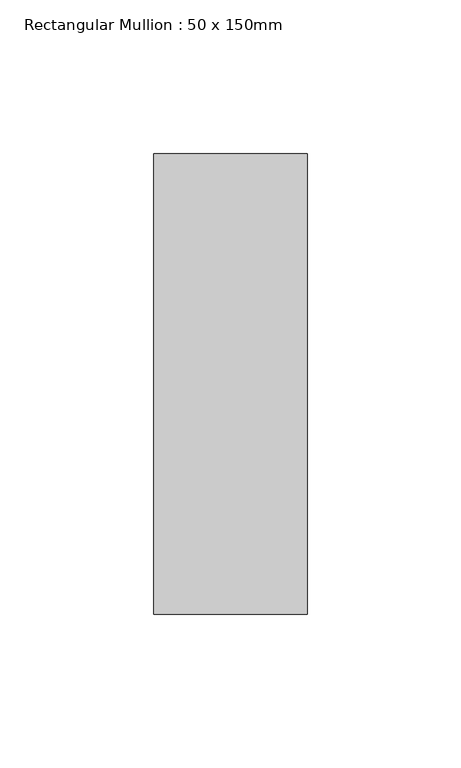
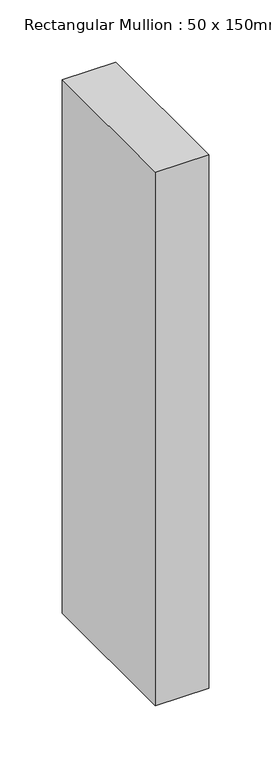
"""IFC4 building model written with IfcOpenShell, lengths in millimetres: member geometry, Rectangular Mullion : 50 x 150mm."""

from ifc_helpers import new_model, si_unit, frame, origin, place, context, project, spatial, polyline, outline, extrude, source, transform, mapped, element, save


def rectangular_mullion_50_x_150mm_5b5377e9(model_context):
    return source(origin(), model_context, "Body", "SweptSolid", [
        extrude(outline(polyline([(0.0, 75.0), (0.0, -75.0), (-50.0, -75.0), (-50.0, 75.0), (0.0, 75.0)])), frame((0.0, 0.0, -525.0), z_axis=(0.0, 0.0, 1.0), x_axis=(1.0, 0.0, 0.0)), (0.0, 0.0, 1.0), 525.0),
    ])


if __name__ == "__main__":
    model = new_model("IFC4")
    model_context = context("Model", 3, world=origin())
    ifc_project = project(units=[si_unit("LENGTHUNIT", "METRE", prefix="MILLI")], contexts=[model_context])
    site = spatial("IfcSite", under=ifc_project)
    building = spatial("IfcBuilding", under=site)
    placement = place(None, origin())
    rectangular_mullion_50_x_150mm_shape = rectangular_mullion_50_x_150mm_5b5377e9(model_context)
    element("IfcMember", 1, ObjectType="Rectangular Mullion : 50 x 150mm", at=placement, inside=building, context=model_context, shape_type="MappedRepresentation", body=[
        mapped(rectangular_mullion_50_x_150mm_shape, transform((0.0, 0.0, 0.0), x_axis=(1.0, 0.0, 0.0), y_axis=(0.0, 1.0, 0.0), z_axis=(0.0, 0.0, 1.0))),
    ])
    save(model, "model.ifc")

# Revit data of these elements
# Type "Rectangular Mullion : 50 x 150mm"
#   built-in parameter 1007304 = 0.492126 (stored number, unit not read)
#   built-in parameter 1007301 = 0.082021 (stored number, unit not read)
#   built-in parameter 1007300 = 0.082021 (stored number, unit not read)
# Element 1 (IfcMember, "Rectangular Mullion : 50 x 150mm")
#   Materials on its faces: "Aluminium"
# Materials
#   "Aluminium": class "Metal", colour RGB 247 247 247, transparency 0, Description = "Aluminium 6061", Cost = 0
